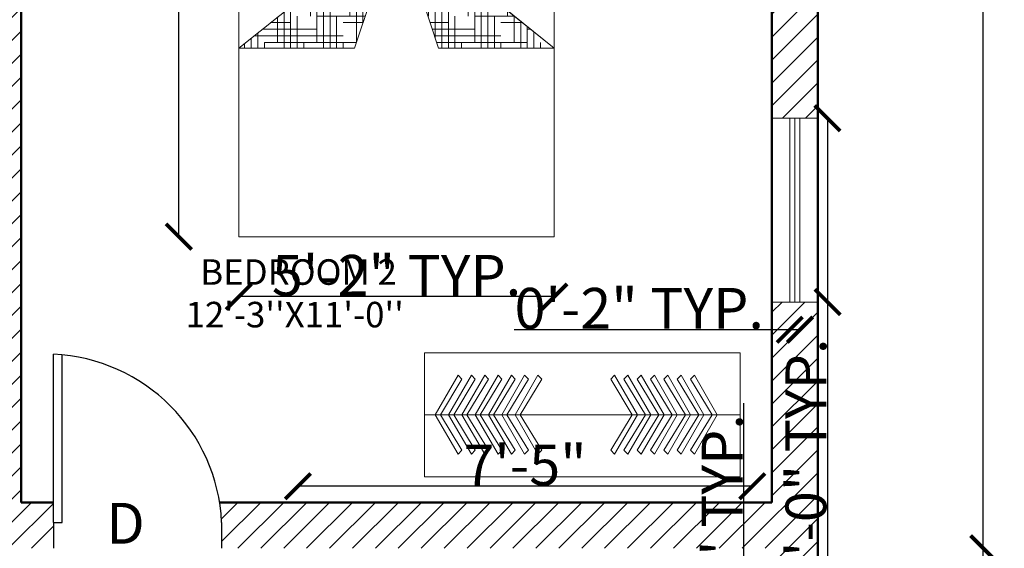
# Model space of a CAD drawing. Units: inches. Extents: x 1385 to 1778, y 1343 to 2100.
# Tile 5 of 6: x 1571 to 1764, y 1821 to 1924. Entities that reach past the tile are written whole.
import ezdxf

# ---------------------------------------------------------------- set-up
doc = ezdxf.new("R2010")
doc.units = ezdxf.units.IN
for name, color, linetype, lineweight in [('A-ANNO-DIMS', 2, 'Continuous', 18), ('A-ANNO-TEXT', 7, 'Continuous', 25), ('A-AREA-IDEN', 7, 'Continuous', 25), ('A-FURN', 8, 'Continuous', 18), ('A-WALL-PATT', 8, 'Continuous', 13), ('Door', 150, 'Continuous', 25), ('Wall', 7, 'Continuous', 50), ('Wardrobe', 114, 'Continuous', 18), ('Windows', 140, 'Continuous', 18)]:
    doc.layers.add(name, color=color, linetype=linetype, lineweight=lineweight)
doc.styles.get("Standard").update_dxf_attribs({"font": 'arial.ttf'})
doc.dimstyles.get("Standard").update_dxf_attribs({"dimtxt": 8, "dimasz": 5, "dimexe": 0.18, "dimexo": 0.0625, "dimgap": 0.09, "dimtad": 1, "dimdec": 1, "dimzin": 0, "dimdsep": 46, "dimlunit": 4, "dimtxsty": 'Standard', "dimblk": 'ARCHTICK', "dimcen": 0.09, "dimse1": 1, "dimse2": 1, "dimadec": 0, "dimazin": 0, "dimtfac": 1, "dimtdec": 1, "dimtofl": 0, "dimtmove": 0, "dimatfit": 3, "dimfxl": 1, "dimtolj": 1, "dimtzin": 0, "dimarcsym": 0})

# ---------------------------------------------------------------- blocks, each defined once
blk = doc.blocks.new('AP0B05')
for p, q in [((35, 100), (35, 880)), ((75, 100), (75, 878.9)), ((35, 100), (35, -20)), ((815, 100), (815, -20))]:
    blk.add_line(p, q)
blk.add_lwpolyline([(35, 100), (75, 100)])
blk.add_arc((-2.4, 62.6), 818.3, 2.6212, 87.3788)
blk = doc.blocks.new('*X10')
at = {"color": 0}
for p, q in [((20.25, 14.8125), (20.2772, 14.8125)), ((20.1739, 14.75), (20.2772, 14.75)), ((20.1875, 14.75), (20.1875, 14.7669)), ((20.199, 14.7812), (20.2772, 14.7812)), ((20.25, 14.3194), (20.25, 14.75)), ((20.1487, 14.7188), (20.2772, 14.7188)), ((20.1562, 14.625), (20.1562, 14.7281)), ((20.0984, 14.6562), (20.125, 14.6562)), ((20.1236, 14.6875), (20.25, 14.6875)), ((20.125, 14.5), (20.125, 14.6893)), ((20.0625, 14.2573), (20.0625, 14.6116)), ((20.0938, 14.375), (20.0938, 14.6504)), ((20.2188, 14.3091), (20.2188, 14.625)), ((20.25, 14.625), (20.2772, 14.625)), ((20.023, 14.5625), (20.2772, 14.5625)), ((20.0312, 14.2469), (20.0312, 14.5727)), ((20.125, 14.5938), (20.2772, 14.5938)), ((19.9979, 14.5312), (20.2772, 14.5312)), ((19.9476, 14.4688), (20.125, 14.4688)), ((19.9727, 14.5), (20.25, 14.5)), ((20, 14.2366), (20, 14.5)), ((20.1875, 14.2987), (20.1875, 14.5)), ((19.9062, 14.375), (19.9062, 14.4174)), ((19.9225, 14.4375), (20, 14.4375)), ((20.25, 14.4375), (20.2772, 14.4375)), ((19.875, 14.25), (19.875, 14.3785)), ((19.9688, 14.2262), (19.9688, 14.375)), ((20, 14.375), (20.2772, 14.375)), ((20.125, 14.4062), (20.2772, 14.4062)), ((20.1562, 14.2884), (20.1562, 14.375)), ((19.8438, 14.1848), (19.8438, 14.3397)), ((19.875, 14.3438), (20.2772, 14.3438)), ((19.7967, 14.2812), (20.125, 14.2812)), ((19.8125, 14.1744), (19.8125, 14.3008)), ((19.8219, 14.3125), (20.2291, 14.3125)), ((19.7716, 14.25), (20, 14.25)), ((19.7812, 14.1641), (19.7812, 14.262)), ((19.9375, 14.2159), (19.9375, 14.25)), ((19.7213, 14.1875), (19.75, 14.1875)), ((19.7465, 14.2188), (19.875, 14.2188)), ((19.75, 14.1537), (19.75, 14.2231)), ((19.7018, 14.0938), (19.7786, 14.0938)), ((19.7188, 14.0726), (19.7188, 14.1136)), ((19.75, 14.0338), (19.75, 14.1032)), ((19.7812, 13.9949), (19.7812, 14.0929)), ((19.7269, 14.0625), (19.8728, 14.0625)), ((19.8125, 14), (19.8125, 14.0825)), ((19.9062, 13.8396), (19.9062, 14.0514)), ((19.752, 14.0312), (19.875, 14.0312)), ((19.875, 13.8784), (19.875, 14)), ((19.9375, 13.8007), (19.9375, 14.0411)), ((19.9688, 13.875), (19.9688, 14.0307)), ((20, 14), (20, 14.0204)), ((20, 14), (20.0614, 14)), ((20.0625, 13.6454), (20.0625, 13.9996)), ((19.875, 13.9688), (20.1557, 13.9688)), ((20.0938, 13.625), (20.0938, 13.9893)), ((20.125, 13.75), (20.125, 13.9789)), ((20.1562, 13.875), (20.1562, 13.9686)), ((19.8275, 13.9375), (20.25, 13.9375)), ((19.8526, 13.9062), (20.125, 13.9062)), ((20.25, 13.5), (20.25, 13.9375)), ((19.8777, 13.875), (20, 13.875)), ((20.0312, 13.6842), (20.0312, 13.875)), ((20.2188, 13.4511), (20.2188, 13.875)), ((20.25, 13.875), (20.2772, 13.875)), ((20, 13.8125), (20.2772, 13.8125)), ((20.125, 13.8438), (20.2772, 13.8438)), ((19.9532, 13.7812), (20.2772, 13.7812)), ((19.9783, 13.75), (20.25, 13.75)), ((20, 13.723), (20, 13.75)), ((20.0035, 13.7188), (20.125, 13.7188)), ((20.1875, 13.49), (20.1875, 13.75)), ((20.25, 13.6875), (20.2772, 13.6875)), ((20.0789, 13.625), (20.2772, 13.625)), ((20.125, 13.6562), (20.2772, 13.6562)), ((20.1562, 13.5288), (20.1562, 13.625)), ((20.104, 13.5938), (20.2772, 13.5938)), ((20.1292, 13.5625), (20.25, 13.5625)), ((20.25, 13.5), (20.2772, 13.5)), ((20.2046, 13.4688), (20.2772, 13.4688)), ((20.2297, 13.4375), (20.2772, 13.4375)), ((20.2549, 13.4062), (20.2772, 13.4062))]:
    blk.add_line(p, q, dxfattribs=at)
blk = doc.blocks.new('MAT-P13')
for p, q in [((-0.75, 0), (0.75, 0)), ((-0.75, 0), (-0.75, -1.9)), ((0.75, 0), (0.75, -1.9)), ((-0.7, -0.05), (-0.7, -0.35)), ((-0.7, -0.05), (-0.05, -0.05)), ((-0.05, -0.35), (-0.05, -0.05)), ((0.05, -0.05), (0.7, -0.05)), ((0.05, -0.35), (0.05, -0.05)), ((0.7, -0.05), (0.7, -0.35)), ((-0.7, -0.35), (-0.05, -0.35)), ((0.05, -0.35), (0.7, -0.35)), ((-0.75, -1.0034), (0, -0.4)), ((0, -0.4), (-0.75, -1.0034)), ((0, -0.4), (-0.2, -1.0034)), ((0, -0.4), (0.2, -1.0034)), ((0, -0.4), (0.75, -1.0034)), ((-0.75, -1.0034), (-0.2, -1.0034)), ((0.2, -1.0034), (0.75, -1.0034)), ((0.75, -1.9), (-0.75, -1.9))]:
    blk.add_line(p, q)
at = {"xscale": -1, "rotation": 90}
blk.add_blockref('*X10', (14.1285, 19.2738), dxfattribs=at)
blk = doc.blocks.new('WARDROBE-DOUBLE')
blk.add_line((0, 12.12), (61.84, 12.12))
blk.add_lwpolyline([(0, 24.24), (61.84, 24.24), (61.84, 0), (0, 0)], close=True)
for points in [[(2.11, 12.12), (6.58, 19.87), (7.34, 19.08), (3.11, 12.12)], [(4.72, 12.12), (9.19, 19.87), (9.95, 19.08), (5.72, 12.12)], [(7.33, 12.12), (11.8, 19.87), (12.56, 19.08), (8.32, 12.12)], [(9.94, 12.12), (14.41, 19.87), (15.17, 19.08), (10.93, 12.12)], [(12.54, 12.12), (17.02, 19.87), (17.78, 19.08), (13.54, 12.12)], [(15.15, 12.12), (19.62, 19.87), (20.38, 19.08), (16.15, 12.12)], [(17.76, 12.12), (22.23, 19.87), (22.99, 19.08), (18.76, 12.12)], [(41.7, 12.12), (37.23, 19.87), (36.47, 19.08), (40.7, 12.12)], [(44.31, 12.12), (39.83, 19.87), (39.07, 19.08), (43.31, 12.12)], [(46.91, 12.12), (42.44, 19.87), (41.68, 19.08), (45.92, 12.12)], [(49.52, 12.12), (45.05, 19.87), (44.29, 19.08), (48.53, 12.12)], [(52.13, 12.12), (47.66, 19.87), (46.9, 19.08), (51.13, 12.12)], [(54.74, 12.12), (50.27, 19.87), (49.51, 19.08), (53.74, 12.12)], [(57.35, 12.12), (52.88, 19.87), (52.12, 19.08), (56.35, 12.12)], [(2.11, 12.12), (6.58, 4.38), (7.34, 5.17), (3.11, 12.12)], [(4.72, 12.12), (9.19, 4.38), (9.95, 5.17), (5.72, 12.12)], [(7.33, 12.12), (11.8, 4.38), (12.56, 5.17), (8.32, 12.12)], [(9.94, 12.12), (14.41, 4.38), (15.17, 5.17), (10.93, 12.12)], [(12.54, 12.12), (17.02, 4.38), (17.78, 5.17), (13.54, 12.12)], [(15.15, 12.12), (19.62, 4.38), (20.38, 5.17), (16.15, 12.12)], [(17.76, 12.12), (22.23, 4.38), (22.99, 5.17), (18.76, 12.12)], [(41.7, 12.12), (37.23, 4.38), (36.47, 5.17), (40.7, 12.12)], [(44.31, 12.12), (39.83, 4.38), (39.07, 5.17), (43.31, 12.12)], [(46.91, 12.12), (42.44, 4.38), (41.68, 5.17), (45.92, 12.12)], [(49.52, 12.12), (45.05, 4.38), (44.29, 5.17), (48.53, 12.12)], [(52.13, 12.12), (47.66, 4.38), (46.9, 5.17), (51.13, 12.12)], [(54.74, 12.12), (50.27, 4.38), (49.51, 5.17), (53.74, 12.12)], [(57.35, 12.12), (52.88, 4.38), (52.12, 5.17), (56.35, 12.12)]]:
    blk.add_lwpolyline(points)
blk = doc.blocks.new('WINDOW-GLAZING-36IN')
for p, q in [((0, 0), (0, 36)), ((1, 0), (1, 36)), ((2, 0), (2, 36))]:
    blk.add_line(p, q)
blk = doc.blocks.new('_ArchTick')
at = {"color": 0, "linetype": 'ByBlock', "const_width": 0.15}
blk.add_lwpolyline([(-0.5, -0.5), (0.5, 0.5)], dxfattribs=at)
blk = doc.blocks.new('*D27')
at = {"layer": 'A-ANNO-DIMS', "color": 0, "lineweight": -2, "transparency": 16777216}
for p, q in [((1729.67, 1904.94), (1729.67, 1868.94)), ((1729.67, 1868.94), (1729.67, 1762.53))]:
    blk.add_line(p, q, dxfattribs=at)
at = {"layer": 'Defpoints', "color": 0, "transparency": 16777216}
for p in [(1724.27, 1904.94), (1724.27, 1868.94), (1729.67, 1868.94)]:
    blk.add_point(p, dxfattribs=at)
at = {"layer": 'A-ANNO-DIMS', "color": 0, "lineweight": -2, "transparency": 16777216, "xscale": 5, "yscale": 5, "zscale": 5}
for p, rotation in [((1729.67, 1904.94), 90), ((1729.67, 1868.94), 270)]:
    blk.add_blockref('_ArchTick', p, dxfattribs=dict(at, rotation=rotation))
at = {"layer": 'A-ANNO-DIMS', "color": 0, "transparency": 16777216, "insert": (1725.44, 1813.24), "char_height": 8, "attachment_point": 5, "rotation": 90}
blk.add_mtext('\\A1;WINDOW 3\'-0" TYP.', dxfattribs=at)
blk = doc.blocks.new('*D28')
at = {"layer": 'A-ANNO-DIMS', "color": 0, "lineweight": -2, "transparency": 16777216}
for p, q in [((1722.27, 1863.54), (1668.33, 1863.54)), ((1724.27, 1863.54), (1722.27, 1863.54))]:
    blk.add_line(p, q, dxfattribs=at)
at = {"layer": 'Defpoints', "color": 0, "transparency": 16777216}
for p in [(1722.27, 1868.94), (1724.27, 1868.94), (1722.27, 1863.54)]:
    blk.add_point(p, dxfattribs=at)
at = {"layer": 'A-ANNO-DIMS', "color": 0, "lineweight": -2, "transparency": 16777216, "xscale": 5, "yscale": 5, "zscale": 5, "rotation": 180}
blk.add_blockref('_ArchTick', (1722.27, 1863.54), dxfattribs=at)
at = {"layer": 'A-ANNO-DIMS', "color": 0, "lineweight": -2, "transparency": 16777216, "xscale": 5, "yscale": 5, "zscale": 5}
blk.add_blockref('_ArchTick', (1724.27, 1863.54), dxfattribs=at)
at = {"layer": 'A-ANNO-DIMS', "color": 0, "transparency": 16777216, "insert": (1692.8, 1867.72), "char_height": 8, "attachment_point": 5}
blk.add_mtext('\\A1;0\'-2" TYP.', dxfattribs=at)
blk = doc.blocks.new('*D31')
at = {"layer": 'A-ANNO-DIMS', "color": 0, "lineweight": -2, "transparency": 16777216}
for p, q in [((1713.27, 1742.73), (1713.27, 1849.15)), ((1713.27, 1682.73), (1713.27, 1742.73))]:
    blk.add_line(p, q, dxfattribs=at)
at = {"layer": 'Defpoints', "color": 0, "transparency": 16777216}
for p in [(1713.27, 1742.73), (1722.27, 1742.73), (1722.27, 1682.73)]:
    blk.add_point(p, dxfattribs=at)
at = {"layer": 'A-ANNO-DIMS', "color": 0, "lineweight": -2, "transparency": 16777216, "xscale": 5, "yscale": 5, "zscale": 5}
for p, rotation in [((1713.27, 1742.73), 90), ((1713.27, 1682.73), 270)]:
    blk.add_blockref('_ArchTick', p, dxfattribs=dict(at, rotation=rotation))
at = {"layer": 'A-ANNO-DIMS', "color": 0, "transparency": 16777216, "insert": (1709.04, 1798.44), "char_height": 8, "attachment_point": 5, "rotation": 90}
blk.add_mtext('\\A1;WINDOW 5\'-0" TYP.', dxfattribs=at)
blk = doc.blocks.new('*D35')
at = {"layer": 'A-ANNO-DIMS', "color": 0, "lineweight": -2, "transparency": 16777216}
for p, q in [((1602.63, 1960.02), (1602.63, 2058.34)), ((1602.63, 1881.75), (1602.63, 1960.02))]:
    blk.add_line(p, q, dxfattribs=at)
at = {"layer": 'Defpoints', "color": 0, "transparency": 16777216}
for p in [(1602.63, 1960.02), (1614.37, 1960.02), (1614.37, 1881.75)]:
    blk.add_point(p, dxfattribs=at)
at = {"layer": 'A-ANNO-DIMS', "color": 0, "lineweight": -2, "transparency": 16777216, "xscale": 5, "yscale": 5, "zscale": 5}
for p, rotation in [((1602.63, 1960.02), 90), ((1602.63, 1881.75), 270)]:
    blk.add_blockref('_ArchTick', p, dxfattribs=dict(at, rotation=rotation))
at = {"layer": 'A-ANNO-DIMS', "color": 0, "transparency": 16777216, "insert": (1598.41, 2011.68), "char_height": 8, "attachment_point": 5, "rotation": 90}
blk.add_mtext('\\A1;BED 6\'-6 1/2" TYP.', dxfattribs=at)
blk = doc.blocks.new('*D36')
at = {"layer": 'A-ANNO-DIMS', "color": 0, "lineweight": -2, "transparency": 16777216}
blk.add_line((1676.17, 1870.01), (1614.37, 1870.01), dxfattribs=at)
at = {"layer": 'Defpoints', "color": 0, "transparency": 16777216}
for p in [(1614.37, 1881.75), (1676.17, 1881.75), (1614.37, 1870.01)]:
    blk.add_point(p, dxfattribs=at)
at = {"layer": 'A-ANNO-DIMS', "color": 0, "lineweight": -2, "transparency": 16777216, "xscale": 5, "yscale": 5, "zscale": 5, "rotation": 180}
blk.add_blockref('_ArchTick', (1614.37, 1870.01), dxfattribs=at)
at = {"layer": 'A-ANNO-DIMS', "color": 0, "lineweight": -2, "transparency": 16777216, "xscale": 5, "yscale": 5, "zscale": 5}
blk.add_blockref('_ArchTick', (1676.17, 1870.01), dxfattribs=at)
at = {"layer": 'A-ANNO-DIMS', "color": 0, "transparency": 16777216, "insert": (1645.27, 1874.18), "char_height": 8, "attachment_point": 5}
blk.add_mtext('\\A1;5\'-2" TYP.', dxfattribs=at)
blk = doc.blocks.new('*D42')
at = {"layer": 'A-ANNO-DIMS', "color": 0, "lineweight": -2, "transparency": 16777216}
blk.add_line((1714.93, 1832.89), (1625.96, 1832.89), dxfattribs=at)
at = {"layer": 'Defpoints', "color": 0, "transparency": 16777216}
for p in [(1625.96, 1832.89), (1625.96, 1816.23), (1714.93, 1816.23)]:
    blk.add_point(p, dxfattribs=at)
at = {"layer": 'A-ANNO-DIMS', "color": 0, "lineweight": -2, "transparency": 16777216, "xscale": 5, "yscale": 5, "zscale": 5, "rotation": 180}
blk.add_blockref('_ArchTick', (1625.96, 1832.89), dxfattribs=at)
at = {"layer": 'A-ANNO-DIMS', "color": 0, "lineweight": -2, "transparency": 16777216, "xscale": 5, "yscale": 5, "zscale": 5}
blk.add_blockref('_ArchTick', (1714.93, 1832.89), dxfattribs=at)
at = {"layer": 'A-ANNO-DIMS', "color": 0, "transparency": 16777216, "insert": (1670.44, 1837.05), "char_height": 8, "attachment_point": 5}
blk.add_mtext('\\A1;7\'-5"', dxfattribs=at)
blk = doc.blocks.new('*D50')
at = {"layer": 'A-ANNO-DIMS', "color": 0, "lineweight": -2, "transparency": 16777216}
blk.add_line((1760.18, 1382.73), (1760.18, 2030.73), dxfattribs=at)
at = {"layer": 'Defpoints', "color": 0, "transparency": 16777216}
for p in [(1727.77, 2030.73), (1760.18, 2030.73), (1727.77, 1382.73)]:
    blk.add_point(p, dxfattribs=at)
at = {"layer": 'A-ANNO-DIMS', "color": 0, "lineweight": -2, "transparency": 16777216, "xscale": 5, "yscale": 5, "zscale": 5}
for p, rotation in [((1760.18, 2030.73), 90), ((1760.18, 1382.73), 270)]:
    blk.add_blockref('_ArchTick', p, dxfattribs=dict(at, rotation=rotation))
at = {"layer": 'A-ANNO-DIMS', "color": 0, "transparency": 16777216, "insert": (1756, 1706.73), "char_height": 8, "attachment_point": 5, "rotation": 90}
blk.add_mtext('\\A1;54\'-0"', dxfattribs=at)
blk = doc.blocks.new('*D54')
at = {"layer": 'A-ANNO-DIMS', "color": 0, "lineweight": -2, "transparency": 16777216}
blk.add_line((1401.37, 1961.73), (1401.37, 1904.94), dxfattribs=at)
at = {"layer": 'Defpoints', "color": 0, "transparency": 16777216}
for p in [(1718.77, 1961.73), (1401.37, 1904.94), (1718.77, 1904.94)]:
    blk.add_point(p, dxfattribs=at)
at = {"layer": 'A-ANNO-DIMS', "color": 0, "lineweight": -2, "transparency": 16777216, "xscale": 5, "yscale": 5, "zscale": 5}
for p, rotation in [((1401.37, 1961.73), 90), ((1401.37, 1904.94), 270)]:
    blk.add_blockref('_ArchTick', p, dxfattribs=dict(at, rotation=rotation))
at = {"layer": 'A-ANNO-DIMS', "color": 0, "transparency": 16777216, "insert": (1397.19, 1933.34), "char_height": 8, "attachment_point": 5, "rotation": 90}
blk.add_mtext('\\A1;4\'-9"', dxfattribs=at)
blk = doc.blocks.new('*D61')
at = {"layer": 'A-ANNO-DIMS', "color": 0, "lineweight": -2, "transparency": 16777216}
blk.add_line((1586.77, 2063.14), (1708.55, 2063.14), dxfattribs=at)
at = {"layer": 'Defpoints', "color": 0, "transparency": 16777216}
for p in [(1708.55, 2063.14), (1586.77, 1382.73), (1708.55, 1382.73)]:
    blk.add_point(p, dxfattribs=at)
at = {"layer": 'A-ANNO-DIMS', "color": 0, "lineweight": -2, "transparency": 16777216, "xscale": 5, "yscale": 5, "zscale": 5, "rotation": 180}
blk.add_blockref('_ArchTick', (1586.77, 2063.14), dxfattribs=at)
at = {"layer": 'A-ANNO-DIMS', "color": 0, "lineweight": -2, "transparency": 16777216, "xscale": 5, "yscale": 5, "zscale": 5}
blk.add_blockref('_ArchTick', (1708.55, 2063.14), dxfattribs=at)
at = {"layer": 'A-ANNO-DIMS', "color": 0, "transparency": 16777216, "insert": (1647.66, 2067.31), "char_height": 8, "attachment_point": 5}
blk.add_mtext('\\A1;10\'-2"', dxfattribs=at)
blk = doc.blocks.new('*D67')
at = {"layer": 'A-ANNO-DIMS', "color": 0, "lineweight": -2, "transparency": 16777216}
for p, q in [((1513.34, 2063.14), (1546.08, 2063.14)), ((1546.08, 2063.14), (1591.31, 2063.14))]:
    blk.add_line(p, q, dxfattribs=at)
at = {"layer": 'Defpoints', "color": 0, "transparency": 16777216}
for p in [(1546.08, 2063.14), (1513.34, 1595.73), (1546.08, 1595.73)]:
    blk.add_point(p, dxfattribs=at)
at = {"layer": 'A-ANNO-DIMS', "color": 0, "lineweight": -2, "transparency": 16777216, "xscale": 5, "yscale": 5, "zscale": 5, "rotation": 180}
blk.add_blockref('_ArchTick', (1513.34, 2063.14), dxfattribs=at)
at = {"layer": 'A-ANNO-DIMS', "color": 0, "lineweight": -2, "transparency": 16777216, "xscale": 5, "yscale": 5, "zscale": 5}
blk.add_blockref('_ArchTick', (1546.08, 2063.14), dxfattribs=at)
at = {"layer": 'A-ANNO-DIMS', "color": 0, "transparency": 16777216, "insert": (1571.19, 2067.37), "char_height": 8, "attachment_point": 5}
blk.add_mtext('\\A1;2\'-8 1/2"', dxfattribs=at)
blk = doc.blocks.new('*D70')
at = {"layer": 'A-ANNO-DIMS', "color": 0, "lineweight": -2, "transparency": 16777216}
for p, q in [((1571.77, 2063.14), (1578.09, 2063.14)), ((1578.09, 2063.14), (1623.18, 2063.14))]:
    blk.add_line(p, q, dxfattribs=at)
at = {"layer": 'Defpoints', "color": 0, "transparency": 16777216}
for p in [(1578.09, 2063.14), (1571.77, 1829.73), (1578.09, 1829.73)]:
    blk.add_point(p, dxfattribs=at)
at = {"layer": 'A-ANNO-DIMS', "color": 0, "lineweight": -2, "transparency": 16777216, "xscale": 5, "yscale": 5, "zscale": 5, "rotation": 180}
blk.add_blockref('_ArchTick', (1571.77, 2063.14), dxfattribs=at)
at = {"layer": 'A-ANNO-DIMS', "color": 0, "lineweight": -2, "transparency": 16777216, "xscale": 5, "yscale": 5, "zscale": 5}
blk.add_blockref('_ArchTick', (1578.09, 2063.14), dxfattribs=at)
at = {"layer": 'A-ANNO-DIMS', "color": 0, "transparency": 16777216, "insert": (1603.14, 2067.37), "char_height": 8, "attachment_point": 5}
blk.add_mtext('\\A1;0\'-6 1/2"', dxfattribs=at)
blk = doc.blocks.new('*D76')
at = {"layer": 'A-ANNO-DIMS', "color": 0, "lineweight": -2, "transparency": 16777216}
for p, q in [((1711.39, 1350.33), (1718.77, 1350.33)), ((1718.77, 1350.33), (1763.86, 1350.33))]:
    blk.add_line(p, q, dxfattribs=at)
at = {"layer": 'Defpoints', "color": 0, "transparency": 16777216}
for p in [(1711.39, 1970.73), (1718.77, 1970.73), (1718.77, 1350.33)]:
    blk.add_point(p, dxfattribs=at)
at = {"layer": 'A-ANNO-DIMS', "color": 0, "lineweight": -2, "transparency": 16777216, "xscale": 5, "yscale": 5, "zscale": 5, "rotation": 180}
blk.add_blockref('_ArchTick', (1711.39, 1350.33), dxfattribs=at)
at = {"layer": 'A-ANNO-DIMS', "color": 0, "lineweight": -2, "transparency": 16777216, "xscale": 5, "yscale": 5, "zscale": 5}
blk.add_blockref('_ArchTick', (1718.77, 1350.33), dxfattribs=at)
at = {"layer": 'A-ANNO-DIMS', "color": 0, "transparency": 16777216, "insert": (1743.82, 1354.56), "char_height": 8, "attachment_point": 5}
blk.add_mtext('\\A1;0\'-7 1/2"', dxfattribs=at)
blk = doc.blocks.new('*D79')
at = {"layer": 'A-ANNO-DIMS', "color": 0, "lineweight": -2, "transparency": 16777216}
blk.add_line((1760.18, 1784.73), (1760.18, 1820.73), dxfattribs=at)
at = {"layer": 'Defpoints', "color": 0, "transparency": 16777216}
for p in [(1508.77, 1820.73), (1760.18, 1820.73), (1508.77, 1784.73)]:
    blk.add_point(p, dxfattribs=at)
at = {"layer": 'A-ANNO-DIMS', "color": 0, "lineweight": -2, "transparency": 16777216, "xscale": 5, "yscale": 5, "zscale": 5}
for p, rotation in [((1760.18, 1820.73), 90), ((1760.18, 1784.73), 270)]:
    blk.add_blockref('_ArchTick', p, dxfattribs=dict(at, rotation=rotation))
at = {"layer": 'A-ANNO-DIMS', "color": 0, "transparency": 16777216, "insert": (1756, 1802.73), "char_height": 8, "attachment_point": 5, "rotation": 90}
blk.add_mtext('\\A1;3\'-0"', dxfattribs=at)

msp = doc.modelspace()

# ---------------------------------------------------------------- hatches: boundary and pattern name
at = {"layer": 'A-WALL-PATT', "transparency": 33554585}
h = msp.add_hatch(dxfattribs=at)
h.set_pattern_fill('ANSI31', color=256)
h.paths.add_polyline_path([(1522.75, 2030.73), (1433.77, 2030.73), (1433.77, 1900.6), (1442.77, 1900.6), (1442.77, 2021.73), (1522.75, 2021.73)])
h.paths.add_polyline_path([(1591.32, 2030.73), (1558.75, 2030.73), (1558.75, 2021.73), (1571.77, 2021.73), (1591.32, 2021.73)], flags=17)
h.paths.add_polyline_path([(1664.16, 2030.73), (1615.32, 2030.73), (1615.32, 2021.73), (1646.77, 2021.73), (1646.77, 1970.73), (1571.77, 1970.73), (1571.77, 1990.51, -0.048507), (1566.67, 1989.78), (1562.77, 1989.78), (1562.77, 1829.73), (1557.76, 1829.73), (1557.76, 1826.48), (1557.76, 1820.73), (1578.09, 1820.73), (1578.09, 1825.8), (1578.09, 1829.73), (1571.77, 1829.73), (1571.77, 1961.73), (1686.02, 1961.73), (1686.02, 1965.64, -0.048507), (1686.76, 1970.73), (1650.77, 1970.73), (1650.77, 2021.73), (1664.16, 2021.73)])
h.paths.add_polyline_path([(1727.77, 2030.73), (1688.16, 2030.73), (1688.16, 2021.73), (1718.77, 2021.73), (1718.77, 1970.73), (1711.39, 1970.73), (1711.39, 1965.64), (1711.39, 1961.73), (1718.77, 1961.73), (1718.77, 1904.94), (1727.77, 1904.94)])
h.paths.add_polyline_path([(1727.77, 1868.94), (1718.77, 1868.94), (1718.77, 1829.73), (1610.61, 1829.73, -0.028655), (1611.02, 1825.8), (1611.02, 1820.73), (1718.77, 1820.73), (1718.77, 1742.73), (1727.77, 1742.73)])
h.paths.add_polyline_path([(1520.45, 1826.48, -0.020905), (1520.74, 1829.73), (1442.77, 1829.73), (1442.77, 1840.6), (1433.77, 1840.6), (1433.77, 1794.33), (1442.77, 1794.33), (1442.77, 1820.73), (1502.77, 1820.73), (1502.77, 1760.73), (1497.07, 1760.73), (1497.07, 1759.8), (1497.07, 1754.73), (1508.77, 1754.73), (1508.77, 1778.73), (1562.77, 1778.73), (1562.77, 1656.82), (1571.77, 1656.82), (1571.77, 1784.73), (1508.77, 1784.73), (1508.77, 1820.73), (1520.45, 1820.73)])
h.paths.add_polyline_path([(1442.77, 1770.33), (1433.77, 1770.33), (1433.77, 1683.46), (1442.77, 1683.46)], flags=17)
h.paths.add_polyline_path([(1656.16, 1603.19, -0.007591), (1656.26, 1604.73), (1622.77, 1604.73), (1622.77, 1595.73), (1656.16, 1595.73)])
h.paths.add_polyline_path([(1727.77, 1682.73), (1718.77, 1682.73), (1718.77, 1604.73), (1704.65, 1604.73), (1704.65, 1603.19), (1704.65, 1595.73), (1727.77, 1595.73)])
h.paths.add_polyline_path([(1513.34, 1595.73), (1513.34, 1604.73), (1442.77, 1604.73), (1442.77, 1647.46), (1433.77, 1647.46), (1433.77, 1531.33), (1442.77, 1531.33), (1442.77, 1595.73)])
h.paths.add_polyline_path([(1546.08, 1604.73), (1546.08, 1595.73), (1577.77, 1595.73), (1577.77, 1472.73), (1541.77, 1472.73), (1541.77, 1523.73), (1537.77, 1523.73), (1537.77, 1472.73), (1442.77, 1472.73), (1442.77, 1495.33), (1433.77, 1495.33), (1433.77, 1382.73), (1586.77, 1382.73), (1586.77, 1391.73), (1442.77, 1391.73), (1442.77, 1463.73), (1586.77, 1463.73), (1586.77, 1604.73)])

# ---------------------------------------------------------------- linework, layer by layer
at = {"layer": 'Wall'}
for p, q in [((1727.77, 2030.73), (1727.77, 1595.73)), ((1571.77, 1961.73), (1571.77, 1829.73)), ((1718.77, 1961.73), (1718.77, 1829.73)), ((1571.77, 1829.73), (1578.09, 1829.73)), ((1610.61, 1829.73), (1718.77, 1829.73))]:
    msp.add_line(p, q, dxfattribs=at)
at = {"layer": 'Windows'}
msp.add_lwpolyline([(1718.77, 1868.94), (1718.77, 1904.94), (1727.77, 1904.94), (1727.77, 1868.94)], close=True, dxfattribs=at)

# ---------------------------------------------------------------- block references
at = {"layer": 'A-FURN', "xscale": -41.19665858361839, "yscale": 41.19665858361839, "zscale": 41.19665858361839}
msp.add_blockref('MAT-P13', (1645.27, 1960.02), dxfattribs=at)
at = {"layer": 'Door', "xscale": 0.0422104207597697, "yscale": 0.0422104207597697, "zscale": 0.0422104207597697}
msp.add_blockref('AP0B05', (1576.61, 1821.58), dxfattribs=at)
at = {"layer": 'Wardrobe'}
msp.add_blockref('WARDROBE-DOUBLE', (1650.74, 1834.76), dxfattribs=at)
at = {"layer": 'Windows', "rotation": 180}
msp.add_blockref('WINDOW-GLAZING-36IN', (1724.27, 1904.94), dxfattribs=at)

# ---------------------------------------------------------------- texts
at = {"layer": 'A-ANNO-TEXT'}
msp.add_text('D', height=8, dxfattribs=at).set_placement((1588.44, 1821.63))
at = {"layer": 'A-AREA-IDEN', "insert": (1600.17, 1877.33), "char_height": 5, "attachment_point": 1}
msp.add_mtext_dynamic_manual_height_columns("\\pxqc; BEDROOM 2\\P12'-3''X11'-0''", width=50.3036, gutter_width=12.5, heights=[0], dxfattribs=at)

# ---------------------------------------------------------------- dimensions: what is measured, and where the dimension line sits
at = {"layer": 'A-ANNO-DIMS'}
for base, p1, p2, picture, middle in [((1546.08, 2063.14), (1513.34, 1595.73), (1546.08, 1595.73), '*D67', (1571.19, 2067.37)), ((1578.09, 2063.14), (1571.77, 1829.73), (1578.09, 1829.73), '*D70', (1603.14, 2067.37)), ((1708.55, 2063.14), (1586.77, 1382.73), (1708.55, 1382.73), '*D61', (1647.66, 2067.31)), ((1718.77, 1350.33), (1711.39, 1970.73), (1718.77, 1970.73), '*D76', (1743.82, 1354.56))]:
    dim = msp.add_linear_dim(base=base, p1=p1, p2=p2, dimstyle='Standard', override={"dimdec": 1, "dimlfac": 1, "dimrnd": 0, "dimzin": 1, "dimdsep": 46, "dimlunit": 4, "dimfrac": 2}, dxfattribs=at)
    dim.commit()
    dim.dimension.update_dxf_attribs({"geometry": picture, "text_midpoint": middle})
for base, p1, p2, angle, text, picture, middle in [((1602.63, 1960.02), (1614.37, 1881.75), (1614.37, 1960.02), 90, 'BED <> TYP.', '*D35', (1598.41, 2011.68)), ((1729.67, 1868.94), (1724.27, 1904.94), (1724.27, 1868.94), 270, 'WINDOW <> TYP.', '*D27', (1725.44, 1813.24)), ((1614.37, 1870.01), (1676.17, 1881.75), (1614.37, 1881.75), 180, '<> TYP.', '*D36', (1645.27, 1874.18)), ((1722.27, 1863.54), (1724.27, 1868.94), (1722.27, 1868.94), 180, '<> TYP.', '*D28', (1692.8, 1867.72)), ((1713.27, 1742.73), (1722.27, 1682.73), (1722.27, 1742.73), 90, 'WINDOW <> TYP.', '*D31', (1709.04, 1798.44))]:
    dim = msp.add_linear_dim(base=base, p1=p1, p2=p2, angle=angle, text=text, dimstyle='Standard', override={"dimdec": 1, "dimlfac": 1, "dimrnd": 0, "dimzin": 1, "dimdsep": 46, "dimlunit": 4, "dimfrac": 2}, dxfattribs=at)
    dim.commit()
    dim.dimension.update_dxf_attribs({"geometry": picture, "text_midpoint": middle})
for base, p1, p2, angle, picture, middle in [((1760.18, 2030.73), (1727.77, 1382.73), (1727.77, 2030.73), 90, '*D50', (1756, 1706.73)), ((1401.37, 1904.94), (1718.77, 1961.73), (1718.77, 1904.94), 90, '*D54', (1397.19, 1933.34)), ((1625.96, 1832.89), (1714.93, 1816.23), (1625.96, 1816.23), 180, '*D42', (1670.44, 1837.05)), ((1760.18, 1820.73), (1508.77, 1784.73), (1508.77, 1820.73), 90, '*D79', (1756, 1802.73))]:
    dim = msp.add_linear_dim(base=base, p1=p1, p2=p2, angle=angle, dimstyle='Standard', override={"dimdec": 1, "dimlfac": 1, "dimrnd": 0, "dimzin": 1, "dimdsep": 46, "dimlunit": 4, "dimfrac": 2}, dxfattribs=at)
    dim.commit()
    dim.dimension.update_dxf_attribs({"geometry": picture, "text_midpoint": middle})

doc.saveas('drawing.dxf')
